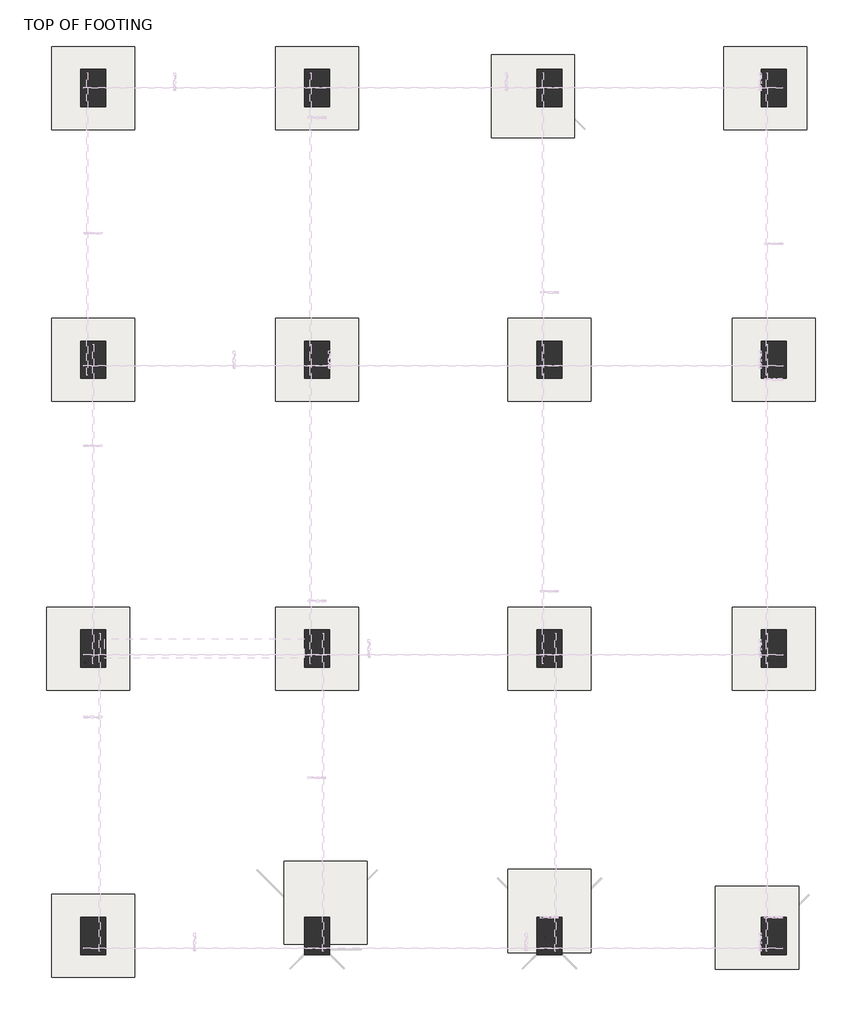
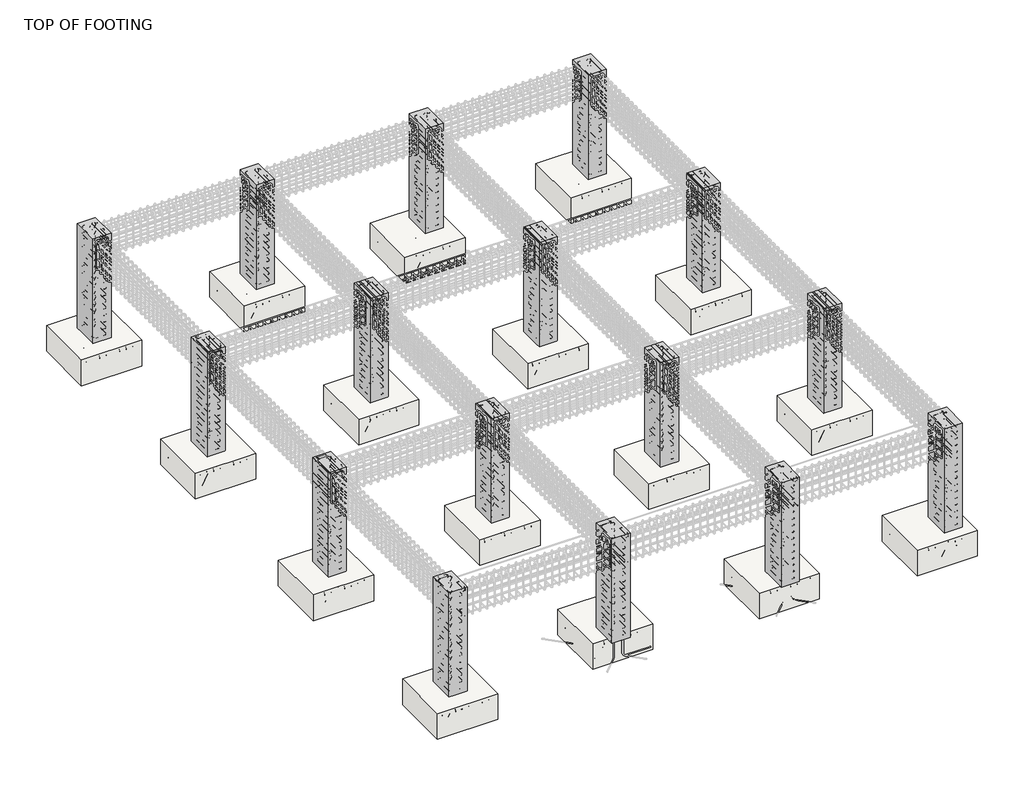
# One storey, part 1 of 14: 16 columns, 16 slabs.
"""IFC4 building model written with IfcOpenShell, lengths in millimetres."""

from ifc_helpers import new_model, si_unit, frame, origin, place, context, project, spatial, polyline, outline, extrude, transform, mapped, element, save
from components import m_footing_rectangular_1000mm_x1000mm_x450mm_4c97ae35

model = new_model("IFC4")

# Units and contexts
model_context = context("Model", 3, world=origin())
ifc_project = project(units=[si_unit("LENGTHUNIT", "METRE", prefix="MILLI")], contexts=[model_context])

# Site, building, storey
site = spatial("IfcSite", under=ifc_project)
building = spatial("IfcBuilding", under=site)
storey = spatial("IfcBuildingStorey", under=building, Name="TOP OF FOOTING", Elevation=-1828.8)

# Columns
placement = place(None, origin())
element("IfcColumn", 1, ObjectType="M_Concrete-Rectangular-Column : 300 x 450mm", at=placement, inside=storey, context=model_context, shape_type="SweptSolid", body=[
    extrude(outline(polyline([(-3307.3533787, 10097.744095), (-3307.3533787, 9647.744095), (-3607.3533787, 9647.744095), (-3607.3533787, 10097.744095), (-3307.3533787, 10097.744095)])), frame((0.0, 0.0, -1828.8), z_axis=(0.0, 0.0, 1.0), x_axis=(1.0, 0.0, 0.0)), (0.0, 0.0, 1.0), 1828.8),
])
element("IfcColumn", 2, ObjectType="M_Concrete-Rectangular-Column : 300 x 450mm", at=placement, inside=storey, context=model_context, shape_type="SweptSolid", body=[
    extrude(outline(polyline([(-607.3533787, 10097.744095), (-607.3533787, 9647.744095), (-907.3533787, 9647.744095), (-907.3533787, 10097.744095), (-607.3533787, 10097.744095)])), frame((0.0, 0.0, -1828.8), z_axis=(0.0, 0.0, 1.0), x_axis=(1.0, 0.0, 0.0)), (0.0, 0.0, 1.0), 1828.8),
])
element("IfcColumn", 3, ObjectType="M_Concrete-Rectangular-Column : 300 x 450mm", at=placement, inside=storey, context=model_context, shape_type="SweptSolid", body=[
    extrude(outline(polyline([(2192.6466213, 10097.744095), (2192.6466213, 9647.744095), (1892.6466213, 9647.744095), (1892.6466213, 10097.744095), (2192.6466213, 10097.744095)])), frame((0.0, 0.0, -1828.8), z_axis=(0.0, 0.0, 1.0), x_axis=(1.0, 0.0, 0.0)), (0.0, 0.0, 1.0), 1828.8),
])
element("IfcColumn", 4, ObjectType="M_Concrete-Rectangular-Column : 300 x 450mm", at=placement, inside=storey, context=model_context, shape_type="SweptSolid", body=[
    extrude(outline(polyline([(4892.6466213, 10097.744095), (4892.6466213, 9647.744095), (4592.6466213, 9647.744095), (4592.6466213, 10097.744095), (4892.6466213, 10097.744095)])), frame((0.0, 0.0, -1828.8), z_axis=(0.0, 0.0, 1.0), x_axis=(1.0, 0.0, 0.0)), (0.0, 0.0, 1.0), 1828.8),
])
element("IfcColumn", 5, ObjectType="M_Concrete-Rectangular-Column : 300 x 450mm", at=placement, inside=storey, context=model_context, shape_type="SweptSolid", body=[
    extrude(outline(polyline([(-3307.3533787, 6826.4938575), (-3307.3533787, 6376.4938575), (-3607.3533787, 6376.4938575), (-3607.3533787, 6826.4938575), (-3307.3533787, 6826.4938575)])), frame((0.0, 0.0, -1828.8), z_axis=(0.0, 0.0, 1.0), x_axis=(1.0, 0.0, 0.0)), (0.0, 0.0, 1.0), 1828.8),
])
element("IfcColumn", 6, ObjectType="M_Concrete-Rectangular-Column : 300 x 450mm", at=placement, inside=storey, context=model_context, shape_type="SweptSolid", body=[
    extrude(outline(polyline([(-607.3533787, 6826.4938575), (-607.3533787, 6376.4938575), (-907.3533787, 6376.4938575), (-907.3533787, 6826.4938575), (-607.3533787, 6826.4938575)])), frame((0.0, 0.0, -1828.8), z_axis=(0.0, 0.0, 1.0), x_axis=(1.0, 0.0, 0.0)), (0.0, 0.0, 1.0), 1828.8),
])
element("IfcColumn", 7, ObjectType="M_Concrete-Rectangular-Column : 300 x 450mm", at=placement, inside=storey, context=model_context, shape_type="SweptSolid", body=[
    extrude(outline(polyline([(2192.6466213, 6826.4938575), (2192.6466213, 6376.4938575), (1892.6466213, 6376.4938575), (1892.6466213, 6826.4938575), (2192.6466213, 6826.4938575)])), frame((0.0, 0.0, -1828.8), z_axis=(0.0, 0.0, 1.0), x_axis=(1.0, 0.0, 0.0)), (0.0, 0.0, 1.0), 1828.8),
])
element("IfcColumn", 8, ObjectType="M_Concrete-Rectangular-Column : 300 x 450mm", at=placement, inside=storey, context=model_context, shape_type="SweptSolid", body=[
    extrude(outline(polyline([(4892.6466213, 6826.4938575), (4892.6466213, 6376.4938575), (4592.6466213, 6376.4938575), (4592.6466213, 6826.4938575), (4892.6466213, 6826.4938575)])), frame((0.0, 0.0, -1828.8), z_axis=(0.0, 0.0, 1.0), x_axis=(1.0, 0.0, 0.0)), (0.0, 0.0, 1.0), 1828.8),
])
element("IfcColumn", 9, ObjectType="M_Concrete-Rectangular-Column : 300 x 450mm", at=placement, inside=storey, context=model_context, shape_type="SweptSolid", body=[
    extrude(outline(polyline([(-3307.3533787, 3349.2498798), (-3307.3533787, 2899.2498798), (-3607.3533787, 2899.2498798), (-3607.3533787, 3349.2498798), (-3307.3533787, 3349.2498798)])), frame((0.0, 0.0, -1828.8), z_axis=(0.0, 0.0, 1.0), x_axis=(1.0, 0.0, 0.0)), (0.0, 0.0, 1.0), 1828.8),
])
element("IfcColumn", 10, ObjectType="M_Concrete-Rectangular-Column : 300 x 450mm", at=placement, inside=storey, context=model_context, shape_type="SweptSolid", body=[
    extrude(outline(polyline([(-607.3533787, 3349.2498798), (-607.3533787, 2899.2498798), (-907.3533787, 2899.2498798), (-907.3533787, 3349.2498798), (-607.3533787, 3349.2498798)])), frame((0.0, 0.0, -1828.8), z_axis=(0.0, 0.0, 1.0), x_axis=(1.0, 0.0, 0.0)), (0.0, 0.0, 1.0), 1828.8),
])
element("IfcColumn", 11, ObjectType="M_Concrete-Rectangular-Column : 300 x 450mm", at=placement, inside=storey, context=model_context, shape_type="SweptSolid", body=[
    extrude(outline(polyline([(2192.6466213, 3349.2498798), (2192.6466213, 2899.2498798), (1892.6466213, 2899.2498798), (1892.6466213, 3349.2498798), (2192.6466213, 3349.2498798)])), frame((0.0, 0.0, -1828.8), z_axis=(0.0, 0.0, 1.0), x_axis=(1.0, 0.0, 0.0)), (0.0, 0.0, 1.0), 1828.8),
])
element("IfcColumn", 12, ObjectType="M_Concrete-Rectangular-Column : 300 x 450mm", at=placement, inside=storey, context=model_context, shape_type="SweptSolid", body=[
    extrude(outline(polyline([(4892.6466213, 3349.2498798), (4892.6466213, 2899.2498798), (4592.6466213, 2899.2498798), (4592.6466213, 3349.2498798), (4892.6466213, 3349.2498798)])), frame((0.0, 0.0, -1828.8), z_axis=(0.0, 0.0, 1.0), x_axis=(1.0, 0.0, 0.0)), (0.0, 0.0, 1.0), 1828.8),
])
element("IfcColumn", 13, ObjectType="M_Concrete-Rectangular-Column : 300 x 450mm", at=placement, inside=storey, context=model_context, shape_type="SweptSolid", body=[
    extrude(outline(polyline([(-3307.3533787, -110.8696759), (-3307.3533787, -560.8696759), (-3607.3533787, -560.8696759), (-3607.3533787, -110.8696759), (-3307.3533787, -110.8696759)])), frame((0.0, 0.0, -1828.8), z_axis=(0.0, 0.0, 1.0), x_axis=(1.0, 0.0, 0.0)), (0.0, 0.0, 1.0), 1828.8),
])
element("IfcColumn", 14, ObjectType="M_Concrete-Rectangular-Column : 300 x 450mm", at=placement, inside=storey, context=model_context, shape_type="SweptSolid", body=[
    extrude(outline(polyline([(-607.3533787, -110.8696759), (-607.3533787, -560.8696759), (-907.3533787, -560.8696759), (-907.3533787, -110.8696759), (-607.3533787, -110.8696759)])), frame((0.0, 0.0, -1828.8), z_axis=(0.0, 0.0, 1.0), x_axis=(1.0, 0.0, 0.0)), (0.0, 0.0, 1.0), 1828.8),
])
element("IfcColumn", 15, ObjectType="M_Concrete-Rectangular-Column : 300 x 450mm", at=placement, inside=storey, context=model_context, shape_type="SweptSolid", body=[
    extrude(outline(polyline([(2192.6466213, -110.8696759), (2192.6466213, -560.8696759), (1892.6466213, -560.8696759), (1892.6466213, -110.8696759), (2192.6466213, -110.8696759)])), frame((0.0, 0.0, -1828.8), z_axis=(0.0, 0.0, 1.0), x_axis=(1.0, 0.0, 0.0)), (0.0, 0.0, 1.0), 1828.8),
])
element("IfcColumn", 16, ObjectType="M_Concrete-Rectangular-Column : 300 x 450mm", at=placement, inside=storey, context=model_context, shape_type="SweptSolid", body=[
    extrude(outline(polyline([(4892.6466213, -110.8696759), (4892.6466213, -560.8696759), (4592.6466213, -560.8696759), (4592.6466213, -110.8696759), (4892.6466213, -110.8696759)])), frame((0.0, 0.0, -1828.8), z_axis=(0.0, 0.0, 1.0), x_axis=(1.0, 0.0, 0.0)), (0.0, 0.0, 1.0), 1828.8),
])

# Slabs
m_footing_rectangular_1000mm_x1000mm_x450mm_shape = m_footing_rectangular_1000mm_x1000mm_x450mm_4c97ae35(model_context)
element("IfcSlab", 17, ObjectType="M_Footing-Rectangular : 1000MM X1000MM X450MM", at=placement, inside=storey, context=model_context, shape_type="MappedRepresentation", body=[
    mapped(m_footing_rectangular_1000mm_x1000mm_x450mm_shape, transform((-3457.3533787, 9872.744095, -1828.8), x_axis=(1.0, 0.0, 0.0), y_axis=(0.0, 1.0, 0.0), z_axis=(0.0, 0.0, 1.0))),
])
element("IfcSlab", 18, ObjectType="M_Footing-Rectangular : 1000MM X1000MM X450MM", at=placement, inside=storey, context=model_context, shape_type="MappedRepresentation", body=[
    mapped(m_footing_rectangular_1000mm_x1000mm_x450mm_shape, transform((-757.3533787, 9872.744095, -1828.8), x_axis=(1.0, 0.0, 0.0), y_axis=(0.0, 1.0, 0.0), z_axis=(0.0, 0.0, 1.0))),
])
element("IfcSlab", 19, ObjectType="M_Footing-Rectangular : 1000MM X1000MM X450MM", at=placement, inside=storey, context=model_context, shape_type="MappedRepresentation", body=[
    mapped(m_footing_rectangular_1000mm_x1000mm_x450mm_shape, transform((1842.6466213, 9772.744095, -1828.8), x_axis=(1.0, 0.0, 0.0), y_axis=(0.0, 1.0, 0.0), z_axis=(0.0, 0.0, 1.0))),
])
element("IfcSlab", 20, ObjectType="M_Footing-Rectangular : 1000MM X1000MM X450MM", at=placement, inside=storey, context=model_context, shape_type="MappedRepresentation", body=[
    mapped(m_footing_rectangular_1000mm_x1000mm_x450mm_shape, transform((4642.6466213, 9872.744095, -1828.8), x_axis=(1.0, 0.0, 0.0), y_axis=(0.0, 1.0, 0.0), z_axis=(0.0, 0.0, 1.0))),
])
element("IfcSlab", 21, ObjectType="M_Footing-Rectangular : 1000MM X1000MM X450MM", at=placement, inside=storey, context=model_context, shape_type="MappedRepresentation", body=[
    mapped(m_footing_rectangular_1000mm_x1000mm_x450mm_shape, transform((-3457.3533787, 6601.4938575, -1828.8), x_axis=(1.0, 0.0, 0.0), y_axis=(0.0, 1.0, 0.0), z_axis=(0.0, 0.0, 1.0))),
])
element("IfcSlab", 22, ObjectType="M_Footing-Rectangular : 1000MM X1000MM X450MM", at=placement, inside=storey, context=model_context, shape_type="MappedRepresentation", body=[
    mapped(m_footing_rectangular_1000mm_x1000mm_x450mm_shape, transform((-757.3533787, 6601.4938575, -1828.8), x_axis=(1.0, 0.0, 0.0), y_axis=(0.0, 1.0, 0.0), z_axis=(0.0, 0.0, 1.0))),
])
element("IfcSlab", 23, ObjectType="M_Footing-Rectangular : 1000MM X1000MM X450MM", at=placement, inside=storey, context=model_context, shape_type="MappedRepresentation", body=[
    mapped(m_footing_rectangular_1000mm_x1000mm_x450mm_shape, transform((2042.6466213, 6601.4938575, -1828.8), x_axis=(1.0, 0.0, 0.0), y_axis=(0.0, 1.0, 0.0), z_axis=(0.0, 0.0, 1.0))),
])
element("IfcSlab", 24, ObjectType="M_Footing-Rectangular : 1000MM X1000MM X450MM", at=placement, inside=storey, context=model_context, shape_type="MappedRepresentation", body=[
    mapped(m_footing_rectangular_1000mm_x1000mm_x450mm_shape, transform((4742.6466213, 6601.4938575, -1828.8), x_axis=(1.0, 0.0, 0.0), y_axis=(0.0, 1.0, 0.0), z_axis=(0.0, 0.0, 1.0))),
])
element("IfcSlab", 25, ObjectType="M_Footing-Rectangular : 1000MM X1000MM X450MM", at=placement, inside=storey, context=model_context, shape_type="MappedRepresentation", body=[
    mapped(m_footing_rectangular_1000mm_x1000mm_x450mm_shape, transform((-3517.3533787, 3124.2498798, -1828.8), x_axis=(1.0, 0.0, 0.0), y_axis=(0.0, 1.0, 0.0), z_axis=(0.0, 0.0, 1.0))),
])
element("IfcSlab", 26, ObjectType="M_Footing-Rectangular : 1000MM X1000MM X450MM", at=placement, inside=storey, context=model_context, shape_type="MappedRepresentation", body=[
    mapped(m_footing_rectangular_1000mm_x1000mm_x450mm_shape, transform((-757.3533787, 3124.2498798, -1828.8), x_axis=(1.0, 0.0, 0.0), y_axis=(0.0, 1.0, 0.0), z_axis=(0.0, 0.0, 1.0))),
])
element("IfcSlab", 27, ObjectType="M_Footing-Rectangular : 1000MM X1000MM X450MM", at=placement, inside=storey, context=model_context, shape_type="MappedRepresentation", body=[
    mapped(m_footing_rectangular_1000mm_x1000mm_x450mm_shape, transform((2042.6466213, 3124.2498798, -1828.8), x_axis=(1.0, 0.0, 0.0), y_axis=(0.0, 1.0, 0.0), z_axis=(0.0, 0.0, 1.0))),
])
element("IfcSlab", 28, ObjectType="M_Footing-Rectangular : 1000MM X1000MM X450MM", at=placement, inside=storey, context=model_context, shape_type="MappedRepresentation", body=[
    mapped(m_footing_rectangular_1000mm_x1000mm_x450mm_shape, transform((4742.6466213, 3124.2498798, -1828.8), x_axis=(1.0, 0.0, 0.0), y_axis=(0.0, 1.0, 0.0), z_axis=(0.0, 0.0, 1.0))),
])
element("IfcSlab", 29, ObjectType="M_Footing-Rectangular : 1000MM X1000MM X450MM", at=placement, inside=storey, context=model_context, shape_type="MappedRepresentation", body=[
    mapped(m_footing_rectangular_1000mm_x1000mm_x450mm_shape, transform((-3457.3533787, -335.8696759, -1828.8), x_axis=(1.0, 0.0, 0.0), y_axis=(0.0, 1.0, 0.0), z_axis=(0.0, 0.0, 1.0))),
])
element("IfcSlab", 30, ObjectType="M_Footing-Rectangular : 1000MM X1000MM X450MM", at=placement, inside=storey, context=model_context, shape_type="MappedRepresentation", body=[
    mapped(m_footing_rectangular_1000mm_x1000mm_x450mm_shape, transform((-657.3533787, 64.1303241, -1828.8), x_axis=(1.0, 0.0, 0.0), y_axis=(0.0, 1.0, 0.0), z_axis=(0.0, 0.0, 1.0))),
])
element("IfcSlab", 31, ObjectType="M_Footing-Rectangular : 1000MM X1000MM X450MM", at=placement, inside=storey, context=model_context, shape_type="MappedRepresentation", body=[
    mapped(m_footing_rectangular_1000mm_x1000mm_x450mm_shape, transform((2042.6466213, -35.8696759, -1828.8), x_axis=(1.0, 0.0, 0.0), y_axis=(0.0, 1.0, 0.0), z_axis=(0.0, 0.0, 1.0))),
])
element("IfcSlab", 32, ObjectType="M_Footing-Rectangular : 1000MM X1000MM X450MM", at=placement, inside=storey, context=model_context, shape_type="MappedRepresentation", body=[
    mapped(m_footing_rectangular_1000mm_x1000mm_x450mm_shape, transform((4542.6466213, -235.8696759, -1828.8), x_axis=(1.0, 0.0, 0.0), y_axis=(0.0, 1.0, 0.0), z_axis=(0.0, 0.0, 1.0))),
])

save(model, "model.ifc")

# Revit data of these elements
# Grids (mm)
#   "1": line (-3457.353, -2084.944) -> (-3457.353, 10642.526)
#   "2": line (-757.353, -2084.944) -> (-757.353, 10642.526)
#   "3": line (2042.647, -2084.944) -> (2042.647, 10642.526)
#   "4": line (4742.647, -2084.944) -> (4742.647, 10642.526)
#   "A": line (7308.665, 9872.744) -> (-4466.682, 9872.744)
#   "B": line (7308.665, 6601.494) -> (-4718.001, 6601.494)
#   "C": line (7308.665, 3124.25) -> (-4585.303, 3124.25)
#   "D": line (6701.92, -335.87) -> (-4307.056, -335.87)
# Type "M_Concrete-Rectangular-Column : 300 x 450mm"
#   b = 300 mm
#   h = 450 mm
#   Structural Material [instance default] = Concrete, Cast-in-Place gray
# Type "M_Footing-Rectangular : 1000MM X1000MM X450MM"
#   Width = 1000 mm
#   Length = 1000 mm
#   Foundation Thickness = 450 mm
#   Structural Material [instance default] = Concrete, Cast-in-Place gray
#   Assembly Code = ""
# Elements 1, 2, 3, 4, 5, 6, 7, 8, 9, 10, 11, 12, 13, 14, 15, 16 (IfcColumn, "M_Concrete-Rectangular-Column : 300 x 450mm")
#   Structural Material = Concrete, Cast-in-Place gray
#   Phase Created = New Construction
#   Materials on its faces: "Concrete, Cast-in-Place gray"
# Elements 17, 18, 19, 20, 21, 22, 23, 24, 25, 26, 27, 28, 29, 30, 31, 32 (IfcSlab, "M_Footing-Rectangular : 1000MM X1000MM X450MM")
#   Structural Material = Concrete, Cast-in-Place gray
#   Phase Created = New Construction
#   Materials on its faces: "Concrete, Cast-in-Place gray"
# Materials
#   "Concrete, Cast-in-Place gray": class "Concrete", colour RGB 192 192 192, transparency 0, Description = "Cast-in-place concrete", Cost = 0
